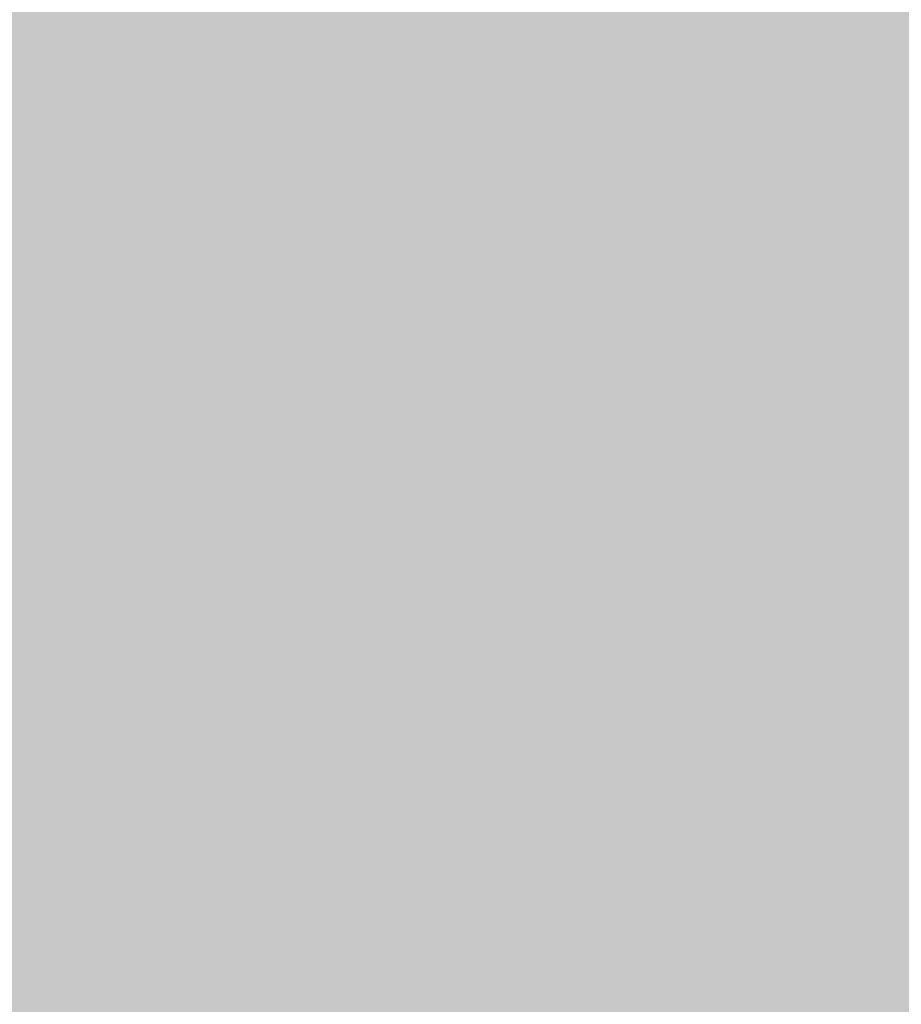
# Model space of a CAD drawing. Units: feet. Extents: x 3168 to 4724, y 827 to 1477.
# Tile 39 of 256: x 3270.273 to 3273.072, y 1093.654 to 1096.781. Entities that reach past the tile are written whole.
import ezdxf

# ---------------------------------------------------------------- set-up
doc = ezdxf.new("R2010")
doc.units = ezdxf.units.FT
doc.layers.add('A-ELEV-PATT', color=8, linetype='Continuous', lineweight=13)

msp = doc.modelspace()

# ---------------------------------------------------------------- hatches: boundary and pattern name
at = {"layer": 'A-ELEV-PATT'}
h = msp.add_hatch(color=256, dxfattribs=at)
h.dxf.hatch_style = 1
edge = h.paths.add_edge_path()
edge.add_ellipse((3552.9058, 979.2201), major_axis=(36.7449, 0), ratio=0.4848485, start_angle=0, end_angle=360)
edge = h.paths.add_edge_path()
edge.add_ellipse((3559.8916, 929.2523), major_axis=(36.7449, 0), ratio=0.4848485, start_angle=0, end_angle=360)
edge = h.paths.add_edge_path()
edge.add_line((3299.3168, 1198.6061), (3479.9167, 1198.6061))
edge.add_line((3479.9167, 1198.6061), (3479.9167, 1209.8686))
edge.add_spline(control_points=[(3479.9167, 1209.8686), (3464.3012, 1209.8686), (3448.6856, 1209.8686), (3410.9491, 1209.8686), (3388.8282, 1209.8686), (3355.6469, 1209.8686), (3344.5864, 1209.8686), (3327.9957, 1209.8686), (3322.4655, 1209.8686), (3314.1702, 1209.8686), (3311.4051, 1209.8686), (3307.2574, 1209.8686), (3305.8748, 1209.8686), (3303.801, 1209.8686), (3303.1097, 1209.8686), (3302.0728, 1209.8686), (3301.7272, 1209.8686), (3301.2087, 1209.8686), (3301.0359, 1209.8686), (3300.7767, 1209.8686), (3300.6903, 1209.8686), (3300.5606, 1209.8686), (3300.5174, 1209.8686), (3300.4526, 1209.8686), (3300.431, 1209.8686), (3300.3986, 1209.8686), (3300.3878, 1209.8686), (3300.3662, 1209.8686), (3300.3457, 1209.8686), (3300.3455, 1209.8686), (3300.3455, 1209.8686), (3300.3433, 1209.8686), (3300.3411, 1209.8686), (3300.3379, 1209.8686), (3300.3368, 1209.8686), (3300.3339, 1209.8686), (3300.3321, 1209.8686), (3300.3255, 1209.8686), (3300.3207, 1209.8686), (3300.3109, 1209.8686), (3300.306, 1209.8686), (3300.2905, 1209.8686), (3300.28, 1209.8686), (3300.2324, 1209.8688), (3300.1953, 1209.869), (3299.9511, 1209.8706), (3299.7448, 1209.8743), (3299.4368, 1209.8833), (3299.3344, 1209.8868), (3299.1811, 1209.8929), (3299.13, 1209.8951), (3298.6522, 1209.9168), (3298.2295, 1209.9457), (3297.6016, 1210.0024), (3297.3934, 1210.0235), (3297.0827, 1210.0583), (3296.9793, 1210.0705), (3296.293, 1210.1549), (3295.7181, 1210.2434), (3294.8687, 1210.3989), (3294.5877, 1210.4545), (3294.1693, 1210.5433), (3294.0304, 1210.5739), (3291.7071, 1211.1012), (3289.6536, 1211.8134), (3285.7763, 1213.564), (3283.9514, 1214.6035), (3280.5122, 1216.9801), (3278.8972, 1218.3176), (3276.3799, 1220.8295), (3275.416, 1221.9177), (3274.0393, 1223.7077), (3273.581, 1224.3495), (3273.1432, 1225.0163)], knot_values=[39.119033, 39.119033, 39.119033, 39.119033, 39.286353, 39.286353, 39.523379, 39.523379, 39.641892, 39.641892, 39.701148, 39.701148, 39.730777, 39.730777, 39.745591, 39.745591, 39.752998, 39.752998, 39.756701, 39.756701, 39.758553, 39.758553, 39.759479, 39.759479, 39.759942, 39.759942, 39.760173, 39.760173, 39.760289, 39.760289, 39.760405, 39.760405, 39.760463, 39.760463, 39.763389, 39.763389, 39.764851, 39.764851, 39.767304, 39.767304, 39.773825, 39.773825, 39.78057, 39.78057, 39.79477, 39.79477, 39.845194, 39.845194, 40.126715, 40.126715, 40.267476, 40.267476, 40.337856, 40.337856, 40.927023, 40.927023, 41.221606, 41.221606, 41.368898, 41.368898, 42.202622, 42.202622, 42.619485, 42.619485, 42.827916, 42.827916, 46.118323, 46.118323, 49.408731, 49.408731, 52.699139, 52.699139, 54.927489, 54.927489, 56.104228, 56.104228, 56.104228, 56.104228], weights=[1, 1, 1, 1, 1, 1, 1, 1, 1, 1, 1, 1, 1, 1, 1, 1, 1, 1, 1, 1, 1, 1, 1, 1, 1, 1, 1, 1, 1, 1, 1, 1, 1, 1, 1, 1, 1, 1, 1, 1, 1, 1, 1, 1, 1, 1, 1, 1, 1, 1, 1, 1, 1, 1, 1, 1, 1, 1, 1, 1, 1, 1, 1, 1, 1, 1, 1, 1, 1, 1, 1, 1, 1, 1], degree=3, periodic=0)
edge.add_line((3273.1432, 1225.0163), (3273.1432, 1099.0163))
edge.add_line((3273.1432, 1099.0163), (3299.3168, 1099.0163))
edge.add_line((3299.3168, 1099.0163), (3299.3168, 1198.6061))
edge = h.paths.add_edge_path()
edge.add_line((3304.7584, 1324.1581), (3479.9167, 1324.1581))
edge.add_line((3479.9167, 1324.1581), (3479.9167, 1335.7146))
edge.add_line((3479.9167, 1335.7146), (3269.1616, 1335.7146))
edge.add_spline(control_points=[(3269.1616, 1335.7146), (3264.0242, 1335.7146), (3258.3641, 1328.9582), (3259.2643, 1323.9003)], knot_values=[0, 0, 0, 0, 15.412191, 15.412191, 15.412191, 15.412191], degree=3, periodic=0)
edge.add_line((3259.2643, 1323.9003), (3265.5168, 1288.7691))
edge.add_line((3265.5168, 1288.7691), (3275.2651, 1261.5456))
edge.add_line((3275.2651, 1261.5456), (3304.7584, 1261.5456))
edge.add_line((3304.7584, 1261.5456), (3304.7584, 1324.1581))
h = msp.add_hatch(color=256, dxfattribs=at)
h.dxf.hatch_style = 1
h.paths.add_polyline_path([(3384.5252, 1099.0163), (3335.0292, 1099.0163), (3299.3168, 1099.0163), (3273.1432, 1099.0163), (3217.5654, 1099.0163), (3168.0693, 827.1163), (3335.0292, 827.1163)])

doc.saveas('drawing.dxf')
